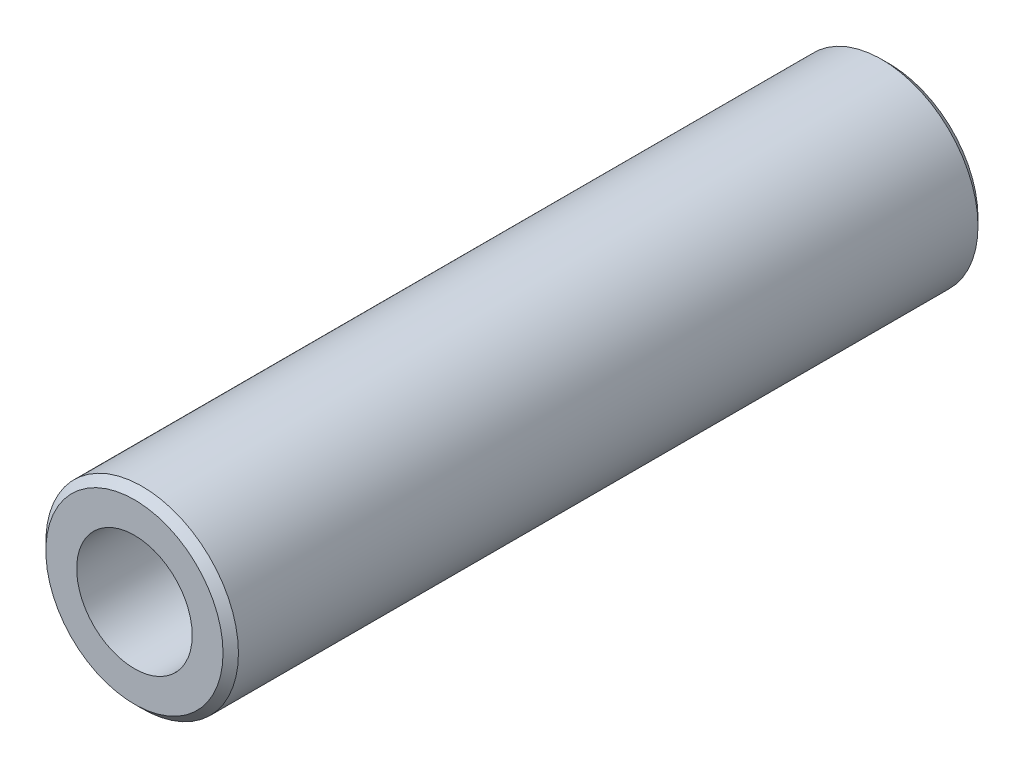
ISO-10303-21;
HEADER;
FILE_DESCRIPTION(('STEP AP214'),'2;1');
FILE_NAME('part.step','',(''),(''),'','','');
FILE_SCHEMA(('AUTOMOTIVE_DESIGN { 1 0 10303 214 1 1 1 1 }'));
ENDSEC;
DATA;
#1=APPLICATION_CONTEXT('core data for automotive mechanical design processes');
#2=APPLICATION_PROTOCOL_DEFINITION('international standard','automotive_design',2000,#1);
#3=PRODUCT_CONTEXT('',#1,'mechanical');
#4=PRODUCT('Part','Part','',(#3));
#5=PRODUCT_RELATED_PRODUCT_CATEGORY('part','',(#4));
#6=PRODUCT_DEFINITION_FORMATION('','',#4);
#7=PRODUCT_DEFINITION_CONTEXT('part definition',#1,'design');
#8=PRODUCT_DEFINITION('design','',#6,#7);
#9=PRODUCT_DEFINITION_SHAPE('','',#8);
#10=(LENGTH_UNIT() NAMED_UNIT(*) SI_UNIT(.MILLI.,.METRE.));
#11=(NAMED_UNIT(*) PLANE_ANGLE_UNIT() SI_UNIT($,.RADIAN.));
#12=(NAMED_UNIT(*) SI_UNIT($,.STERADIAN.) SOLID_ANGLE_UNIT());
#13=UNCERTAINTY_MEASURE_WITH_UNIT(LENGTH_MEASURE(1.E-05),#10,'distance_accuracy_value','');
#14=(GEOMETRIC_REPRESENTATION_CONTEXT(3) GLOBAL_UNCERTAINTY_ASSIGNED_CONTEXT((#13)) GLOBAL_UNIT_ASSIGNED_CONTEXT((#10,
#11,#12)) REPRESENTATION_CONTEXT('',''));
#15=CARTESIAN_POINT('',(0.,0.,0.));
#16=DIRECTION('',(0.,0.,1.));
#17=DIRECTION('',(1.,0.,0.));
#18=AXIS2_PLACEMENT_3D('',#15,#16,#17);
#19=CARTESIAN_POINT('',(0.,0.,24.5));
#20=DIRECTION('',(0.,0.,1.));
#21=DIRECTION('',(1.,0.,0.));
#22=AXIS2_PLACEMENT_3D('',#19,#20,#21);
#23=PLANE('',#22);
#24=CARTESIAN_POINT('',(0.,0.,24.5));
#25=DIRECTION('',(0.,0.,1.));
#26=DIRECTION('',(1.,0.,0.));
#27=AXIS2_PLACEMENT_3D('',#24,#25,#26);
#28=CIRCLE('',#27,5.75);
#29=CARTESIAN_POINT('',(5.75,0.,24.5));
#30=VERTEX_POINT('',#29);
#31=EDGE_CURVE('E11',#30,#30,#28,.T.);
#32=ORIENTED_EDGE('',*,*,#31,.T.);
#33=EDGE_LOOP('',(#32));
#34=FACE_BOUND('',#33,.T.);
#35=CARTESIAN_POINT('',(0.,0.,24.5));
#36=DIRECTION('',(0.,0.,1.));
#37=DIRECTION('',(1.,0.,0.));
#38=AXIS2_PLACEMENT_3D('',#35,#36,#37);
#39=CIRCLE('',#38,3.75);
#40=CARTESIAN_POINT('',(3.75,0.,24.5));
#41=VERTEX_POINT('',#40);
#42=EDGE_CURVE('E69',#41,#41,#39,.T.);
#43=ORIENTED_EDGE('',*,*,#42,.F.);
#44=EDGE_LOOP('',(#43));
#45=FACE_BOUND('',#44,.T.);
#46=ADVANCED_FACE('F47',(#34,#45),#23,.T.);
#47=CARTESIAN_POINT('',(0.,0.,-24.5));
#48=DIRECTION('',(0.,0.,1.));
#49=DIRECTION('',(1.,0.,0.));
#50=AXIS2_PLACEMENT_3D('',#47,#48,#49);
#51=PLANE('',#50);
#52=CARTESIAN_POINT('',(0.,0.,-24.5));
#53=DIRECTION('',(0.,0.,1.));
#54=DIRECTION('',(1.,0.,0.));
#55=AXIS2_PLACEMENT_3D('',#52,#53,#54);
#56=CIRCLE('',#55,5.74999999999998);
#57=CARTESIAN_POINT('',(5.74999999999998,0.,-24.5));
#58=VERTEX_POINT('',#57);
#59=EDGE_CURVE('E60',#58,#58,#56,.F.);
#60=ORIENTED_EDGE('',*,*,#59,.T.);
#61=EDGE_LOOP('',(#60));
#62=FACE_BOUND('',#61,.T.);
#63=CARTESIAN_POINT('',(0.,0.,-24.5));
#64=DIRECTION('',(0.,0.,1.));
#65=DIRECTION('',(1.,0.,0.));
#66=AXIS2_PLACEMENT_3D('',#63,#64,#65);
#67=CIRCLE('',#66,3.75);
#68=CARTESIAN_POINT('',(3.75,0.,-24.5));
#69=VERTEX_POINT('',#68);
#70=EDGE_CURVE('E72',#69,#69,#67,.T.);
#71=ORIENTED_EDGE('',*,*,#70,.T.);
#72=EDGE_LOOP('',(#71));
#73=FACE_BOUND('',#72,.T.);
#74=ADVANCED_FACE('F81',(#62,#73),#51,.F.);
#75=CARTESIAN_POINT('',(0.,0.,24.5));
#76=DIRECTION('',(0.,0.,-1.));
#77=DIRECTION('',(-1.,0.,0.));
#78=AXIS2_PLACEMENT_3D('',#75,#76,#77);
#79=CYLINDRICAL_SURFACE('',#78,6.25);
#80=CARTESIAN_POINT('',(0.,0.,-24.));
#81=DIRECTION('',(0.,0.,1.));
#82=DIRECTION('',(1.,0.,0.));
#83=AXIS2_PLACEMENT_3D('',#80,#81,#82);
#84=CIRCLE('',#83,6.25);
#85=CARTESIAN_POINT('',(6.25,0.,-24.));
#86=VERTEX_POINT('',#85);
#87=EDGE_CURVE('E64',#86,#86,#84,.T.);
#88=ORIENTED_EDGE('',*,*,#87,.T.);
#89=EDGE_LOOP('',(#88));
#90=FACE_BOUND('',#89,.T.);
#91=CARTESIAN_POINT('',(0.,0.,24.));
#92=DIRECTION('',(0.,0.,1.));
#93=DIRECTION('',(1.,0.,0.));
#94=AXIS2_PLACEMENT_3D('',#91,#92,#93);
#95=CIRCLE('',#94,6.25);
#96=CARTESIAN_POINT('',(6.25,0.,24.));
#97=VERTEX_POINT('',#96);
#98=EDGE_CURVE('E62',#97,#97,#95,.F.);
#99=ORIENTED_EDGE('',*,*,#98,.T.);
#100=EDGE_LOOP('',(#99));
#101=FACE_BOUND('',#100,.T.);
#102=ADVANCED_FACE('F87',(#90,#101),#79,.T.);
#103=CARTESIAN_POINT('',(0.,0.,24.5));
#104=DIRECTION('',(0.,0.,-1.));
#105=DIRECTION('',(-1.,0.,0.));
#106=AXIS2_PLACEMENT_3D('',#103,#104,#105);
#107=CYLINDRICAL_SURFACE('',#106,3.75);
#108=ORIENTED_EDGE('',*,*,#42,.T.);
#109=EDGE_LOOP('',(#108));
#110=FACE_BOUND('',#109,.T.);
#111=ORIENTED_EDGE('',*,*,#70,.F.);
#112=EDGE_LOOP('',(#111));
#113=FACE_BOUND('',#112,.T.);
#114=ADVANCED_FACE('F76',(#110,#113),#107,.F.);
#115=CARTESIAN_POINT('',(0.,0.,-24.));
#116=DIRECTION('',(0.,0.,1.));
#117=DIRECTION('',(1.,0.,0.));
#118=AXIS2_PLACEMENT_3D('',#115,#116,#117);
#119=CONICAL_SURFACE('',#118,6.25,0.785398163397454);
#120=ORIENTED_EDGE('',*,*,#59,.F.);
#121=EDGE_LOOP('',(#120));
#122=FACE_BOUND('',#121,.T.);
#123=ORIENTED_EDGE('',*,*,#87,.F.);
#124=EDGE_LOOP('',(#123));
#125=FACE_BOUND('',#124,.T.);
#126=ADVANCED_FACE('F94',(#122,#125),#119,.T.);
#127=CARTESIAN_POINT('',(0.,0.,24.5));
#128=DIRECTION('',(0.,0.,-1.));
#129=DIRECTION('',(-1.,0.,0.));
#130=AXIS2_PLACEMENT_3D('',#127,#128,#129);
#131=CONICAL_SURFACE('',#130,5.75,0.785398163397447);
#132=ORIENTED_EDGE('',*,*,#98,.F.);
#133=EDGE_LOOP('',(#132));
#134=FACE_BOUND('',#133,.T.);
#135=ORIENTED_EDGE('',*,*,#31,.F.);
#136=EDGE_LOOP('',(#135));
#137=FACE_BOUND('',#136,.T.);
#138=ADVANCED_FACE('F55',(#134,#137),#131,.T.);
#139=CLOSED_SHELL('',(#46,#74,#102,#114,#126,#138));
#140=MANIFOLD_SOLID_BREP('B2',#139);
#141=ADVANCED_BREP_SHAPE_REPRESENTATION('',(#18,#140),#14);
#142=SHAPE_DEFINITION_REPRESENTATION(#9,#141);
ENDSEC;
END-ISO-10303-21;
